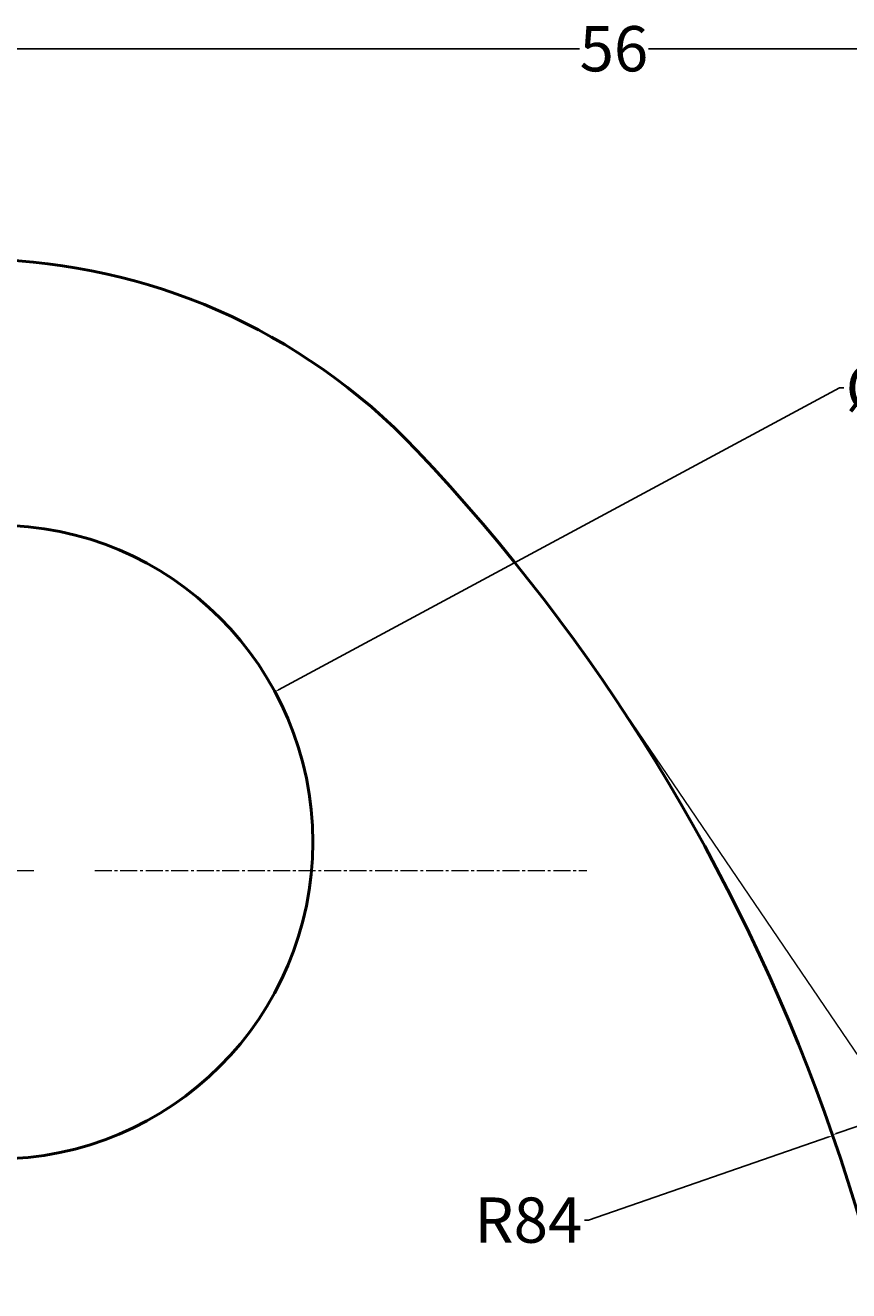
# Model space of a CAD drawing. Units: millimetres. Extents: x -60 to 113, y -37 to 126.
# Tile 15 of 17: x 13 to 49, y 70 to 126. Entities that reach past the tile are written whole.
import ezdxf

# ---------------------------------------------------------------- set-up
doc = ezdxf.new("R2010")
doc.units = ezdxf.units.MM
doc.header["$MEASUREMENT"] = 0
doc.linetypes.add('CENTER2', pattern=[1.125, 0.75, -0.125, 0.125, -0.125])
for name, color, linetype, lineweight in [('M-CNTR', 4, 'CENTER2', 18), ('M-CONS', 8, 'Continuous', 13), ('M-DIMS', 2, 'Continuous', 25), ('M-OUTL', 7, 'Continuous', 50)]:
    doc.layers.add(name, color=color, linetype=linetype, lineweight=lineweight)
doc.styles.get("Standard").update_dxf_attribs({"font": 'arial.ttf'})
doc.dimstyles.get("Standard").update_dxf_attribs({"dimtxt": 0.18, "dimasz": 0.18, "dimexe": 0.18, "dimexo": 0.0625, "dimgap": 0.09, "dimtad": 0, "dimtih": 1, "dimtoh": 1, "dimdec": 4, "dimzin": 0, "dimdsep": 46, "dimtxsty": 'Standard', "dimcen": 0.09, "dimadec": 0, "dimazin": 0, "dimtfac": 1, "dimtdec": 4, "dimtofl": 0, "dimtmove": 0, "dimatfit": 3, "dimfxl": 1, "dimtolj": 1, "dimtzin": 0, "dimarcsym": 0})

# ---------------------------------------------------------------- blocks, each defined once
blk = doc.blocks.new('*U1')
at = {"layer": 'M-CNTR', "color": 0, "transparency": 16777216}
for p, q in [((0, 5.4), (0, 27.12)), ((-27.12, 0), (-5.4, 0)), ((5.4, 0), (27.12, 0)), ((0, -27.12), (0, -5.4))]:
    blk.add_line(p, q, dxfattribs=at)
at = {"layer": 'M-CNTR', "color": 0, "linetype": 'Continuous', "transparency": 16777216}
for p, q in [((0, -2.7), (0, 2.7)), ((-2.7, 0), (2.7, 0))]:
    blk.add_line(p, q, dxfattribs=at)
blk = doc.blocks.new('*D7')
at = {"layer": 'Defpoints', "color": 0, "transparency": 16777216}
for p in [(48.606, 76.822), (-30.775, 49.351)]:
    blk.add_point(p, dxfattribs=at)
at = {"layer": 'M-DIMS', "color": 0, "lineweight": -2, "transparency": 16777216}
for p, q in [((37.821, 73.09), (48.435, 76.764)), ((37.641, 73.09), (37.821, 73.09))]:
    blk.add_line(p, q, dxfattribs=at)
at = {"layer": 'M-DIMS', "color": 0, "transparency": 16777216}
blk.add_solid([(48.426, 76.792), (48.445, 76.735), (48.606, 76.822)], dxfattribs=at)
at = {"layer": 'M-DIMS', "color": 0, "transparency": 16777216, "insert": (35.165, 73.09), "char_height": 0.18, "attachment_point": 5}
blk.add_mtext('\\A1;{\\H11.11111x;R84}', dxfattribs=at)
blk = doc.blocks.new('*D8')
at = {"layer": 'Defpoints', "color": 0, "transparency": 16777216}
for p in [(23.977, 96.423), (-0.678, 83.151)]:
    blk.add_point(p, dxfattribs=at)
at = {"layer": 'M-DIMS', "color": 0, "lineweight": -2, "transparency": 16777216}
for p, q in [((48.912, 109.846), (24.135, 96.508)), ((49.092, 109.846), (48.912, 109.846)), ((11.559, 89.787), (11.739, 89.787)), ((11.649, 89.697), (11.649, 89.877))]:
    blk.add_line(p, q, dxfattribs=at)
at = {"layer": 'M-DIMS', "color": 0, "transparency": 16777216}
blk.add_solid([(24.121, 96.535), (24.149, 96.482), (23.977, 96.423)], dxfattribs=at)
at = {"layer": 'M-DIMS', "color": 0, "transparency": 16777216, "insert": (51.704, 109.846), "char_height": 0.18, "attachment_point": 5}
blk.add_mtext('\\A1;{\\H11.11111x;%%C28}', dxfattribs=at)
blk = doc.blocks.new('*D17')
at = {"layer": 'Defpoints', "color": 0, "transparency": 16777216}
for p in [(67.355, 124.823), (10.532, 88.533), (67.355, 6.442)]:
    blk.add_point(p, dxfattribs=at)
at = {"layer": 'M-DIMS', "color": 0, "lineweight": -2, "transparency": 16777216}
for p, q in [((10.532, 88.595), (10.532, 125.003)), ((10.712, 124.823), (37.422, 124.823)), ((67.175, 124.823), (40.465, 124.823)), ((67.355, 6.504), (67.355, 125.003))]:
    blk.add_line(p, q, dxfattribs=at)
at = {"layer": 'M-DIMS', "color": 0, "transparency": 16777216}
for points in [[(10.712, 124.853), (10.712, 124.793), (10.532, 124.823)], [(67.175, 124.853), (67.175, 124.793), (67.355, 124.823)]]:
    blk.add_solid(points, dxfattribs=at)
at = {"layer": 'M-DIMS', "color": 0, "transparency": 16777216, "insert": (38.944, 124.823), "char_height": 0.18, "attachment_point": 5}
blk.add_mtext('\\A1;{\\H11.11111x;56}', dxfattribs=at)
blk = doc.blocks.new('HOLE-D28')
blk.add_circle((14, 14), 14)
blk = doc.blocks.new('*D24')
at = {"layer": 'Defpoints', "color": 0, "transparency": 16777216}
for p in [(48.596, 76.851), (-30.775, 49.351)]:
    blk.add_point(p, dxfattribs=at)
at = {"layer": 'M-DIMS', "color": 0, "lineweight": -2, "transparency": 16777216}
for p, q in [((96.218, 93.35), (48.766, 76.909)), ((96.398, 93.35), (96.218, 93.35)), ((-30.865, 49.351), (-30.685, 49.351)), ((-30.775, 49.261), (-30.775, 49.441))]:
    blk.add_line(p, q, dxfattribs=at)
at = {"layer": 'M-DIMS', "color": 0, "transparency": 16777216}
blk.add_solid([(48.756, 76.938), (48.776, 76.881), (48.596, 76.851)], dxfattribs=at)
at = {"layer": 'M-DIMS', "color": 0, "transparency": 16777216, "insert": (97.018, 93.35), "char_height": 0.18, "attachment_point": 5}
blk.add_mtext('\\A1;R84.0000', dxfattribs=at)

msp = doc.modelspace()

# ---------------------------------------------------------------- linework, layer by layer
at = {"layer": 'M-CONS'}
msp.add_line((38.71594, 96.54155), (89.53778, 21.70335), dxfattribs=at)
at = {"layer": 'M-OUTL'}
for centre, radius, start, end in [((10.62227, 88.53289), 27, 43.425324, 223.425324), ((-30.77517, 49.3506), 84, 356.2470441, 43.4253235)]:
    msp.add_arc(centre, radius, start, end, dxfattribs=at)

# ---------------------------------------------------------------- block references
at = {"layer": 'M-CNTR'}
msp.add_blockref('*U1', (10.62227, 88.53289), dxfattribs=at)
at = {"layer": 'M-OUTL'}
msp.add_blockref('HOLE-D28', (-2.3502, 75.7872), dxfattribs=at)

# ---------------------------------------------------------------- dimensions: what is measured, and where the dimension line sits
at = {"layer": 'M-DIMS'}
dim = msp.add_linear_dim(base=(67.35481, 124.82251), p1=(10.53227, 88.53289), p2=(67.35481, 6.44179), text='{\\H11.11111x;56}', dimstyle='Standard', override={"dimclrd": 0, "dimclre": 0, "dimclrt": 0}, dxfattribs=at)
dim.commit()
dim.dimension.update_dxf_attribs({"geometry": '*D17', "text_midpoint": (38.94354, 124.82251)})
dim = msp.add_diameter_dim_2p(p1=(-0.67791, 83.1508), p2=(23.97668, 96.423), text='{\\H11.11111x;%%C28}', dimstyle='Standard', override={"dimclrd": 0, "dimclre": 0, "dimclrt": 0}, dxfattribs=at)
dim.commit()
dim.dimension.update_dxf_attribs({"geometry": '*D8', "text_midpoint": (51.70419, 109.84614), "dimtype": 163})
dim = msp.add_radius_dim(center=(-30.77517, 49.3506), mpoint=(48.59582, 76.85052), dimstyle='Standard', override={"dimdec": 4, "dimlfac": 1, "dimrnd": 0, "dimzin": 0, "dimdsep": 46, "dimlunit": 2}, dxfattribs=at)
dim.commit()
dim.dimension.update_dxf_attribs({"geometry": '*D24', "text_midpoint": (97.01779, 93.35047), "dimtype": 164})
dim = msp.add_radius_dim(center=(-30.77517, 49.3506), mpoint=(48.60556, 76.82239), text='{\\H11.11111x;R84}', dimstyle='Standard', override={"dimclrd": 0, "dimclre": 0, "dimclrt": 0}, dxfattribs=at)
dim.commit()
dim.dimension.update_dxf_attribs({"geometry": '*D7', "text_midpoint": (35.16548, 73.09007), "dimtype": 164})

doc.saveas('drawing.dxf')
